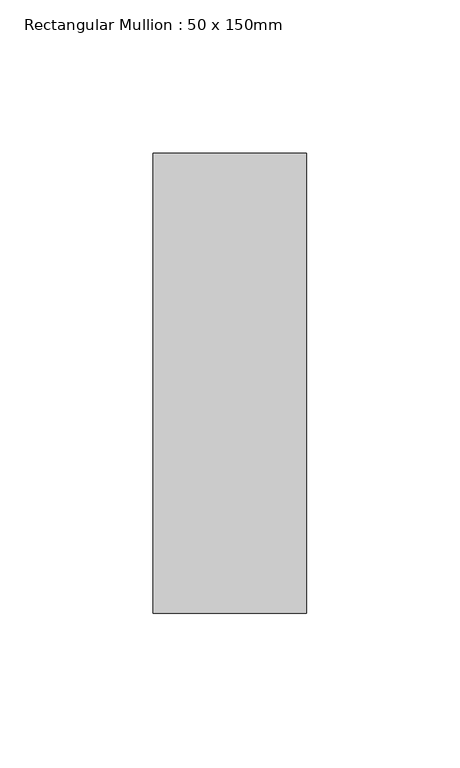
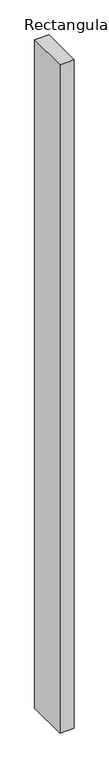
"""IFC4 building model written with IfcOpenShell, lengths in millimetres: member geometry, Rectangular Mullion : 50 x 150mm."""

from ifc_helpers import new_model, si_unit, frame, origin, place, context, project, spatial, polyline, outline, extrude, source, transform, mapped, element, save


def rectangular_mullion_50_x_150mm_4a8db126(model_context):
    return source(origin(), model_context, "Body", "SweptSolid", [
        extrude(outline(polyline([(0.0, 75.0), (0.0, -75.0), (-50.0, -75.0), (-50.0, 75.0), (0.0, 75.0)])), frame((0.0, 0.0, -2438.4), z_axis=(0.0, 0.0, 1.0), x_axis=(1.0, 0.0, 0.0)), (0.0, 0.0, 1.0), 2438.4),
    ])


if __name__ == "__main__":
    model = new_model("IFC4")
    model_context = context("Model", 3, world=origin())
    ifc_project = project(units=[si_unit("LENGTHUNIT", "METRE", prefix="MILLI")], contexts=[model_context])
    site = spatial("IfcSite", under=ifc_project)
    building = spatial("IfcBuilding", under=site)
    placement = place(None, origin())
    rectangular_mullion_50_x_150mm_shape = rectangular_mullion_50_x_150mm_4a8db126(model_context)
    element("IfcMember", 1, ObjectType="Rectangular Mullion : 50 x 150mm", at=placement, inside=building, context=model_context, shape_type="MappedRepresentation", body=[
        mapped(rectangular_mullion_50_x_150mm_shape, transform((0.0, 0.0, 0.0), x_axis=(1.0, 0.0, 0.0), y_axis=(0.0, 1.0, 0.0), z_axis=(0.0, 0.0, 1.0))),
    ])
    save(model, "model.ifc")

# Revit data of these elements
# Type "Rectangular Mullion : 50 x 150mm"
#   built-in parameter 1007304 = 0.492126 (stored number, unit not read)
#   built-in parameter 1007301 = 0.082021 (stored number, unit not read)
#   built-in parameter 1007300 = 0.082021 (stored number, unit not read)
# Element 1 (IfcMember, "Rectangular Mullion : 50 x 150mm")
#   Materials on its faces: "Aluminium"
# Materials
#   "Aluminium": class "Metal", colour RGB 247 247 247, transparency 0, Description = "Aluminium 6061", Cost = 0
